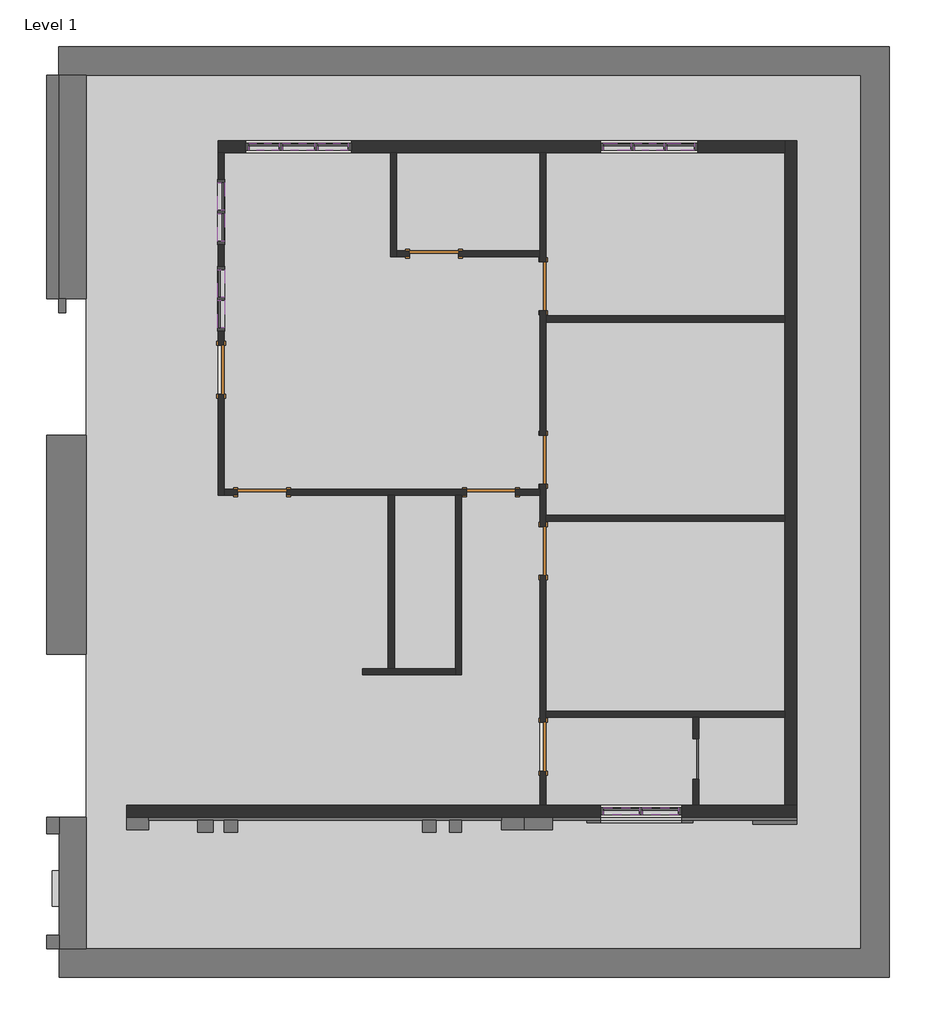
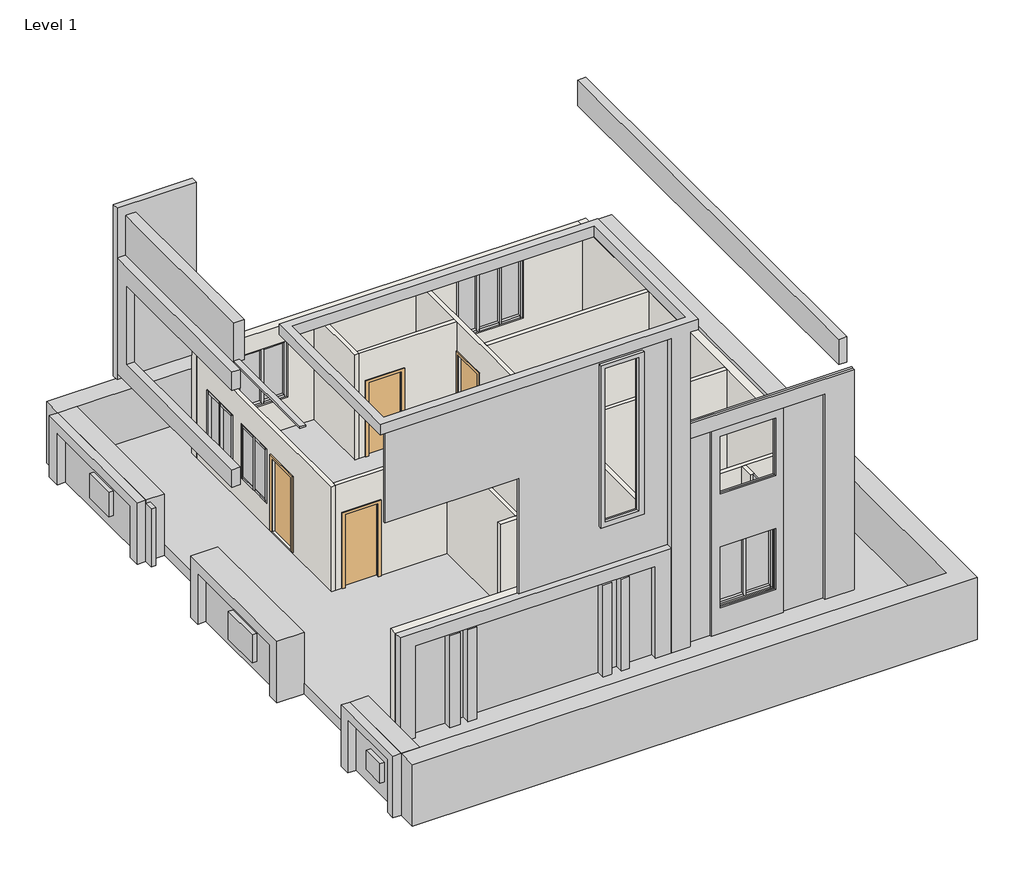
# One storey: 41 members, 15 walls, 13 plates, 8 doors, 7 proxies.
"""IFC4 building model written with IfcOpenShell, lengths in millimetres."""

from ifc_helpers import new_model, si_unit, frame, origin, origin_with_axes, place, context, project, spatial, polyline, outline, extrude, faceted_brep, transform, mapped, element, save
from components import generic_models_1_generic_models_1_e43304c4, generic_models_10_generic_models_10_cbb95902, generic_models_3_generic_models_3_0e3346f0, generic_models_4_generic_models_4_c94f5d84, generic_models_5_generic_models_5_fcb812c2, generic_models_6_generic_models_6_7d9998ff, generic_models_8_generic_models_8_478b8fa0, door_305aa2a5, door_e5f9f3c4, member_0b7646a3, member_1fe8360d, member_921b0d60, member_90febb00, member_2e0784aa, member_a400357f, member_a980948f, member_6f432376, member_c6b50b9a, member_293a584d, member_16047d0f, member_00baf460, member_c33c434a, member_eeabd68d, member_85079546, system_panel_glazed_353c4472, system_panel_glazed_f9beff23, system_panel_glazed_2aec2d59, system_panel_glazed_df895792, system_panel_glazed_ced102d0, system_panel_glazed_0ced4b38, system_panel_glazed_3427ea54, system_panel_glazed_7f229d02

model = new_model("IFC4")

# Units and contexts
model_context = context("Model", 3, world=origin())
ifc_project = project(units=[si_unit("LENGTHUNIT", "METRE", prefix="MILLI")], contexts=[model_context])

# Site, building, storey
site = spatial("IfcSite", under=ifc_project)
building = spatial("IfcBuilding", under=site)
storey = spatial("IfcBuildingStorey", under=building, Name="Level 1", Elevation=0.0)

# Proxies
placement = place(None, origin())
generic_models_1_generic_models_1_shape = generic_models_1_generic_models_1_e43304c4(model_context)
element("IfcBuildingElementProxy", 1, Name="Generic Models 1 : Generic Models 1", ObjectType="Generic Models 1 : Generic Models 1", at=placement, inside=storey, context=model_context, shape_type="MappedRepresentation", body=[
    mapped(generic_models_1_generic_models_1_shape, transform((0.0, 0.0, 0.0), x_axis=(1.0, 0.0, 0.0), y_axis=(0.0, 1.0, 0.0), z_axis=(0.0, 0.0, 1.0))),
])
generic_models_10_generic_models_10_shape = generic_models_10_generic_models_10_cbb95902(model_context)
element("IfcBuildingElementProxy", 2, Name="Generic Models 10 : Generic Models 10", ObjectType="Generic Models 10 : Generic Models 10", at=placement, inside=storey, context=model_context, shape_type="MappedRepresentation", body=[
    mapped(generic_models_10_generic_models_10_shape, transform((0.0, 0.0, 0.0), x_axis=(1.0, 0.0, 0.0), y_axis=(0.0, 1.0, 0.0), z_axis=(0.0, 0.0, 1.0))),
])
generic_models_3_generic_models_3_shape = generic_models_3_generic_models_3_0e3346f0(model_context)
element("IfcBuildingElementProxy", 3, Name="Generic Models 3 : Generic Models 3", ObjectType="Generic Models 3 : Generic Models 3", at=placement, inside=storey, context=model_context, shape_type="MappedRepresentation", body=[
    mapped(generic_models_3_generic_models_3_shape, transform((0.0, 0.0, 0.0), x_axis=(1.0, 0.0, 0.0), y_axis=(0.0, 1.0, 0.0), z_axis=(0.0, 0.0, 1.0))),
])
generic_models_4_generic_models_4_shape = generic_models_4_generic_models_4_c94f5d84(model_context)
element("IfcBuildingElementProxy", 4, Name="Generic Models 4 : Generic Models 4", ObjectType="Generic Models 4 : Generic Models 4", at=placement, inside=storey, context=model_context, shape_type="MappedRepresentation", body=[
    mapped(generic_models_4_generic_models_4_shape, transform((0.0, 0.0, 0.0), x_axis=(1.0, 0.0, 0.0), y_axis=(0.0, 1.0, 0.0), z_axis=(0.0, 0.0, 1.0))),
])
generic_models_5_generic_models_5_shape = generic_models_5_generic_models_5_fcb812c2(model_context)
element("IfcBuildingElementProxy", 5, Name="Generic Models 5 : Generic Models 5", ObjectType="Generic Models 5 : Generic Models 5", at=placement, inside=storey, context=model_context, shape_type="MappedRepresentation", body=[
    mapped(generic_models_5_generic_models_5_shape, transform((0.0, 0.0, 0.0), x_axis=(1.0, 0.0, 0.0), y_axis=(0.0, 1.0, 0.0), z_axis=(0.0, 0.0, 1.0))),
])
generic_models_6_generic_models_6_shape = generic_models_6_generic_models_6_7d9998ff(model_context)
element("IfcBuildingElementProxy", 6, Name="Generic Models 6 : Generic Models 6", ObjectType="Generic Models 6 : Generic Models 6", at=placement, inside=storey, context=model_context, shape_type="MappedRepresentation", body=[
    mapped(generic_models_6_generic_models_6_shape, transform((0.0, 0.0, 0.0), x_axis=(1.0, 0.0, 0.0), y_axis=(0.0, 1.0, 0.0), z_axis=(0.0, 0.0, 1.0))),
])
generic_models_8_generic_models_8_shape = generic_models_8_generic_models_8_478b8fa0(model_context)
element("IfcBuildingElementProxy", 7, Name="Generic Models 8 : Generic Models 8", ObjectType="Generic Models 8 : Generic Models 8", at=placement, inside=storey, context=model_context, shape_type="MappedRepresentation", body=[
    mapped(generic_models_8_generic_models_8_shape, transform((0.0, 0.0, 0.0), x_axis=(1.0, 0.0, 0.0), y_axis=(0.0, 1.0, 0.0), z_axis=(0.0, 0.0, 1.0))),
])

# Doors
door_shape = door_305aa2a5(model_context)
element("IfcDoor", 8, ObjectType="Single-Flush : 36\" x 84\"", at=placement, inside=storey, context=model_context, shape_type="MappedRepresentation", body=[
    mapped(door_shape, transform((-18378.8003587, -5510.4026331, 50.8), x_axis=(0.0, 1.0, 0.0), y_axis=(-1.0, 0.0, 0.0), z_axis=(0.0, 0.0, 1.0))),
])
element("IfcDoor", 9, ObjectType="Single-Flush : 36\" x 84\"", at=placement, inside=storey, context=model_context, shape_type="MappedRepresentation", body=[
    mapped(door_shape, transform((-17616.8003587, -7796.4026331, 0.0), x_axis=(-1.0, 0.0, 0.0), y_axis=(0.0, -1.0, 0.0), z_axis=(0.0, 0.0, 1.0))),
])
element("IfcDoor", 10, ObjectType="Single-Flush : 36\" x 84\"", at=placement, inside=storey, context=model_context, shape_type="MappedRepresentation", body=[
    mapped(door_shape, transform((-14397.3503587, -3338.7026331, 0.0), x_axis=(-1.0, 0.0, 0.0), y_axis=(0.0, -1.0, 0.0), z_axis=(0.0, 0.0, 1.0))),
])
element("IfcDoor", 11, ObjectType="Single-Flush : 36\" x 84\"", at=placement, inside=storey, context=model_context, shape_type="MappedRepresentation", body=[
    mapped(door_shape, transform((-13330.5503587, -7796.4026331, 0.0), x_axis=(-1.0, 0.0, 0.0), y_axis=(0.0, -1.0, 0.0), z_axis=(0.0, 0.0, 1.0))),
])
element("IfcDoor", 12, ObjectType="Single-Flush : 36\" x 84\"", at=placement, inside=storey, context=model_context, shape_type="MappedRepresentation", body=[
    mapped(door_shape, transform((-12359.0003587, -8894.9526331, 0.0), x_axis=(0.0, 1.0, 0.0), y_axis=(-1.0, 0.0, 0.0), z_axis=(0.0, 0.0, 1.0))),
])
element("IfcDoor", 13, ObjectType="Single-Flush : 36\" x 84\"", at=placement, inside=storey, context=model_context, shape_type="MappedRepresentation", body=[
    mapped(door_shape, transform((-12359.0003587, -12552.5526331, 76.2), x_axis=(0.0, 1.0, 0.0), y_axis=(-1.0, 0.0, 0.0), z_axis=(0.0, 0.0, 1.0))),
])
door_2_shape = door_e5f9f3c4(model_context)
element("IfcDoor", 14, ObjectType="Single-Flush : 36\" x 84\"", at=placement, inside=storey, context=model_context, shape_type="MappedRepresentation", body=[
    mapped(door_2_shape, transform((-12359.0003587, -3948.3026331, 0.0), x_axis=(0.0, -1.0, 0.0), y_axis=(1.0, 0.0, 0.0), z_axis=(0.0, 0.0, 1.0))),
])
element("IfcDoor", 15, ObjectType="Single-Flush : 36\" x 84\"", at=placement, inside=storey, context=model_context, shape_type="MappedRepresentation", body=[
    mapped(door_2_shape, transform((-12359.0003587, -7186.8026331, 0.0), x_axis=(0.0, -1.0, 0.0), y_axis=(1.0, 0.0, 0.0), z_axis=(0.0, 0.0, 1.0))),
])

# Members
member_shape = member_0b7646a3(model_context)
element("IfcMember", 16, ObjectType="Rectangular Mullion : 2.5\" x 5\" rectangular", at=placement, inside=storey, context=model_context, shape_type="MappedRepresentation", body=[
    mapped(member_shape, transform((-18378.8003587, -2525.9026331, 2289.8702949), x_axis=(0.0, 0.0, 1.0), y_axis=(-1.0, 0.0, 0.0), z_axis=(0.0, -1.0, 0.0))),
])
element("IfcMember", 17, ObjectType="Rectangular Mullion : 2.5\" x 5\" rectangular", at=placement, inside=storey, context=model_context, shape_type="MappedRepresentation", body=[
    mapped(member_shape, transform((-18378.8003587, -3103.7526331, 2289.8702949), x_axis=(0.0, 0.0, 1.0), y_axis=(-1.0, 0.0, 0.0), z_axis=(0.0, -1.0, 0.0))),
])
element("IfcMember", 18, ObjectType="Rectangular Mullion : 2.5\" x 5\" rectangular", at=placement, inside=storey, context=model_context, shape_type="MappedRepresentation", body=[
    mapped(member_shape, transform((-18378.8003587, -4212.3782104, 2289.8702949), x_axis=(0.0, 0.0, 1.0), y_axis=(1.0, 0.0, 0.0), z_axis=(0.0, 1.0, 0.0))),
])
element("IfcMember", 19, ObjectType="Rectangular Mullion : 2.5\" x 5\" rectangular", at=placement, inside=storey, context=model_context, shape_type="MappedRepresentation", body=[
    mapped(member_shape, transform((-18378.8003587, -3634.5282104, 2289.8702949), x_axis=(0.0, 0.0, 1.0), y_axis=(1.0, 0.0, 0.0), z_axis=(0.0, 1.0, 0.0))),
])
element("IfcMember", 20, ObjectType="Rectangular Mullion : 2.5\" x 5\" rectangular", at=placement, inside=storey, context=model_context, shape_type="MappedRepresentation", body=[
    mapped(member_shape, transform((-10714.3503587, -1338.4526331, 2669.0215701), x_axis=(0.0, 0.0, 1.0), y_axis=(0.0, -1.0, 0.0), z_axis=(1.0, 0.0, 0.0))),
])
element("IfcMember", 21, ObjectType="Rectangular Mullion : 2.5\" x 5\" rectangular", at=placement, inside=storey, context=model_context, shape_type="MappedRepresentation", body=[
    mapped(member_shape, transform((-9526.9003587, -1338.4526331, 2669.0215701), x_axis=(0.0, 0.0, 1.0), y_axis=(0.0, -1.0, 0.0), z_axis=(1.0, 0.0, 0.0))),
])
member_2_shape = member_1fe8360d(model_context)
element("IfcMember", 22, ObjectType="Rectangular Mullion : 2.5\" x 5\" rectangular", at=placement, inside=storey, context=model_context, shape_type="MappedRepresentation", body=[
    mapped(member_2_shape, transform((-18378.8003587, -2557.6526331, 812.6731894), x_axis=(0.0, -1.0, 0.0), y_axis=(-1.0, 0.0, 0.0), z_axis=(0.0, 0.0, -1.0))),
])
element("IfcMember", 23, ObjectType="Rectangular Mullion : 2.5\" x 5\" rectangular", at=placement, inside=storey, context=model_context, shape_type="MappedRepresentation", body=[
    mapped(member_shape, transform((-18378.8003587, -2589.4026331, 812.6731894), x_axis=(0.0, 0.0, -1.0), y_axis=(-1.0, 0.0, 0.0), z_axis=(0.0, 1.0, 0.0))),
])
element("IfcMember", 24, ObjectType="Rectangular Mullion : 2.5\" x 5\" rectangular", at=placement, inside=storey, context=model_context, shape_type="MappedRepresentation", body=[
    mapped(member_shape, transform((-18378.8003587, -2011.5526331, 812.6731894), x_axis=(0.0, 0.0, -1.0), y_axis=(-1.0, 0.0, 0.0), z_axis=(0.0, 1.0, 0.0))),
])
element("IfcMember", 25, ObjectType="Rectangular Mullion : 2.5\" x 5\" rectangular", at=placement, inside=storey, context=model_context, shape_type="MappedRepresentation", body=[
    mapped(member_shape, transform((-18378.8003587, -4148.8782104, 718.4753468), x_axis=(0.0, 0.0, -1.0), y_axis=(1.0, 0.0, 0.0), z_axis=(0.0, -1.0, 0.0))),
])
element("IfcMember", 26, ObjectType="Rectangular Mullion : 2.5\" x 5\" rectangular", at=placement, inside=storey, context=model_context, shape_type="MappedRepresentation", body=[
    mapped(member_shape, transform((-18378.8003587, -4726.7282104, 718.4753468), x_axis=(0.0, 0.0, -1.0), y_axis=(1.0, 0.0, 0.0), z_axis=(0.0, -1.0, 0.0))),
])
element("IfcMember", 27, ObjectType="Rectangular Mullion : 2.5\" x 5\" rectangular", at=placement, inside=storey, context=model_context, shape_type="MappedRepresentation", body=[
    mapped(member_shape, transform((-10041.2503587, -1338.4526331, 927.2562283), x_axis=(0.0, 0.0, -1.0), y_axis=(0.0, -1.0, 0.0), z_axis=(-1.0, 0.0, 0.0))),
])
element("IfcMember", 28, ObjectType="Rectangular Mullion : 2.5\" x 5\" rectangular", at=placement, inside=storey, context=model_context, shape_type="MappedRepresentation", body=[
    mapped(member_shape, transform((-11228.7003587, -1338.4526331, 927.2562283), x_axis=(0.0, 0.0, -1.0), y_axis=(0.0, -1.0, 0.0), z_axis=(-1.0, 0.0, 0.0))),
])
member_3_shape = member_921b0d60(model_context)
element("IfcMember", 29, ObjectType="Rectangular Mullion : 2.5\" x 5\" rectangular", at=placement, inside=storey, context=model_context, shape_type="MappedRepresentation", body=[
    mapped(member_3_shape, transform((-18378.8003587, -3167.2526331, 812.6731894), x_axis=(0.0, -1.0, 0.0), y_axis=(-1.0, 0.0, 0.0), z_axis=(0.0, 0.0, -1.0))),
])
element("IfcMember", 30, ObjectType="Rectangular Mullion : 2.5\" x 5\" rectangular", at=placement, inside=storey, context=model_context, shape_type="MappedRepresentation", body=[
    mapped(member_3_shape, transform((-18378.8003587, -1948.0526331, 2289.8702949), x_axis=(0.0, 1.0, 0.0), y_axis=(-1.0, 0.0, 0.0), z_axis=(0.0, 0.0, 1.0))),
])
member_4_shape = member_90febb00(model_context)
element("IfcMember", 31, ObjectType="Rectangular Mullion : 2.5\" x 5\" rectangular", at=placement, inside=storey, context=model_context, shape_type="MappedRepresentation", body=[
    mapped(member_4_shape, transform((-18378.8003587, -4180.6282104, 718.4753468), x_axis=(0.0, 1.0, 0.0), y_axis=(1.0, 0.0, 0.0), z_axis=(0.0, 0.0, -1.0))),
])
member_5_shape = member_2e0784aa(model_context)
element("IfcMember", 32, ObjectType="Rectangular Mullion : 2.5\" x 5\" rectangular", at=placement, inside=storey, context=model_context, shape_type="MappedRepresentation", body=[
    mapped(member_5_shape, transform((-18378.8003587, -4790.2282104, 2289.8702949), x_axis=(0.0, -1.0, 0.0), y_axis=(1.0, 0.0, 0.0), z_axis=(0.0, 0.0, 1.0))),
])
element("IfcMember", 33, ObjectType="Rectangular Mullion : 2.5\" x 5\" rectangular", at=placement, inside=storey, context=model_context, shape_type="MappedRepresentation", body=[
    mapped(member_5_shape, transform((-18378.8003587, -3571.0282104, 718.4753468), x_axis=(0.0, 1.0, 0.0), y_axis=(1.0, 0.0, 0.0), z_axis=(0.0, 0.0, -1.0))),
])
member_6_shape = member_a400357f(model_context)
element("IfcMember", 34, ObjectType="Rectangular Mullion : 2.5\" x 5\" rectangular", at=placement, inside=storey, context=model_context, shape_type="MappedRepresentation", body=[
    mapped(member_6_shape, transform((-16632.5503587, -1338.4526331, 2544.0832428), x_axis=(0.0, 0.0, 1.0), y_axis=(0.0, -1.0, 0.0), z_axis=(1.0, 0.0, 0.0))),
])
element("IfcMember", 35, ObjectType="Rectangular Mullion : 2.5\" x 5\" rectangular", at=placement, inside=storey, context=model_context, shape_type="MappedRepresentation", body=[
    mapped(member_6_shape, transform((-17229.4503587, -1338.4526331, 900.2328231), x_axis=(0.0, 0.0, -1.0), y_axis=(0.0, -1.0, 0.0), z_axis=(-1.0, 0.0, 0.0))),
])
member_7_shape = member_a980948f(model_context)
element("IfcMember", 36, ObjectType="Rectangular Mullion : 2.5\" x 5\" rectangular", at=placement, inside=storey, context=model_context, shape_type="MappedRepresentation", body=[
    mapped(member_7_shape, transform((-10104.7503587, -1338.4526331, 2669.0215701), x_axis=(0.0, 0.0, 1.0), y_axis=(0.0, -1.0, 0.0), z_axis=(1.0, 0.0, 0.0))),
])
element("IfcMember", 37, ObjectType="Rectangular Mullion : 2.5\" x 5\" rectangular", at=placement, inside=storey, context=model_context, shape_type="MappedRepresentation", body=[
    mapped(member_7_shape, transform((-10650.8503587, -1338.4526331, 927.2562283), x_axis=(0.0, 0.0, -1.0), y_axis=(0.0, -1.0, 0.0), z_axis=(-1.0, 0.0, 0.0))),
])
member_8_shape = member_6f432376(model_context)
element("IfcMember", 38, ObjectType="Rectangular Mullion : 2.5\" x 5\" rectangular", at=placement, inside=storey, context=model_context, shape_type="MappedRepresentation", body=[
    mapped(member_8_shape, transform((-17292.9503587, -1338.4526331, 2544.0832428), x_axis=(0.0, 0.0, 1.0), y_axis=(0.0, -1.0, 0.0), z_axis=(1.0, 0.0, 0.0))),
])
element("IfcMember", 39, ObjectType="Rectangular Mullion : 2.5\" x 5\" rectangular", at=placement, inside=storey, context=model_context, shape_type="MappedRepresentation", body=[
    mapped(member_8_shape, transform((-16003.9003587, -1338.4526331, 2544.0832428), x_axis=(0.0, 0.0, 1.0), y_axis=(0.0, -1.0, 0.0), z_axis=(1.0, 0.0, 0.0))),
])
element("IfcMember", 40, ObjectType="Rectangular Mullion : 2.5\" x 5\" rectangular", at=placement, inside=storey, context=model_context, shape_type="MappedRepresentation", body=[
    mapped(member_8_shape, transform((-16569.0503587, -1338.4526331, 900.2328231), x_axis=(0.0, 0.0, -1.0), y_axis=(0.0, -1.0, 0.0), z_axis=(-1.0, 0.0, 0.0))),
])
element("IfcMember", 41, ObjectType="Rectangular Mullion : 2.5\" x 5\" rectangular", at=placement, inside=storey, context=model_context, shape_type="MappedRepresentation", body=[
    mapped(member_8_shape, transform((-17858.1003587, -1338.4526331, 900.2328231), x_axis=(0.0, 0.0, -1.0), y_axis=(0.0, -1.0, 0.0), z_axis=(-1.0, 0.0, 0.0))),
])
member_9_shape = member_c6b50b9a(model_context)
element("IfcMember", 42, ObjectType="Rectangular Mullion : 2.5\" x 5\" rectangular", at=placement, inside=storey, context=model_context, shape_type="MappedRepresentation", body=[
    mapped(member_9_shape, transform((-10682.6003587, -1338.4526331, 927.2562283), x_axis=(1.0, 0.0, 0.0), y_axis=(0.0, -1.0, 0.0), z_axis=(0.0, 0.0, -1.0))),
])
element("IfcMember", 43, ObjectType="Rectangular Mullion : 2.5\" x 5\" rectangular", at=placement, inside=storey, context=model_context, shape_type="MappedRepresentation", body=[
    mapped(member_9_shape, transform((-10073.0003587, -1338.4526331, 927.2562283), x_axis=(1.0, 0.0, 0.0), y_axis=(0.0, -1.0, 0.0), z_axis=(0.0, 0.0, -1.0))),
])
member_10_shape = member_293a584d(model_context)
element("IfcMember", 44, ObjectType="Rectangular Mullion : 2.5\" x 5\" rectangular", at=placement, inside=storey, context=model_context, shape_type="MappedRepresentation", body=[
    mapped(member_10_shape, transform((-11292.2003587, -1338.4526331, 2669.0215701), x_axis=(-1.0, 0.0, 0.0), y_axis=(0.0, -1.0, 0.0), z_axis=(0.0, 0.0, 1.0))),
])
element("IfcMember", 45, ObjectType="Rectangular Mullion : 2.5\" x 5\" rectangular", at=placement, inside=storey, context=model_context, shape_type="MappedRepresentation", body=[
    mapped(member_10_shape, transform((-9463.4003587, -1338.4526331, 927.2562283), x_axis=(1.0, 0.0, 0.0), y_axis=(0.0, -1.0, 0.0), z_axis=(0.0, 0.0, -1.0))),
])
member_11_shape = member_16047d0f(model_context)
element("IfcMember", 46, ObjectType="Rectangular Mullion : 2.5\" x 5\" rectangular", at=placement, inside=storey, context=model_context, shape_type="MappedRepresentation", body=[
    mapped(member_11_shape, transform((-16600.8003587, -1338.4526331, 900.2328231), x_axis=(1.0, 0.0, 0.0), y_axis=(0.0, -1.0, 0.0), z_axis=(0.0, 0.0, -1.0))),
])
element("IfcMember", 47, ObjectType="Rectangular Mullion : 2.5\" x 5\" rectangular", at=placement, inside=storey, context=model_context, shape_type="MappedRepresentation", body=[
    mapped(member_11_shape, transform((-17261.2003587, -1338.4526331, 900.2328231), x_axis=(1.0, 0.0, 0.0), y_axis=(0.0, -1.0, 0.0), z_axis=(0.0, 0.0, -1.0))),
])
member_12_shape = member_00baf460(model_context)
element("IfcMember", 48, ObjectType="Rectangular Mullion : 2.5\" x 5\" rectangular", at=placement, inside=storey, context=model_context, shape_type="MappedRepresentation", body=[
    mapped(member_12_shape, transform((-17921.6003587, -1338.4526331, 2544.0832428), x_axis=(-1.0, 0.0, 0.0), y_axis=(0.0, -1.0, 0.0), z_axis=(0.0, 0.0, 1.0))),
])
element("IfcMember", 49, ObjectType="Rectangular Mullion : 2.5\" x 5\" rectangular", at=placement, inside=storey, context=model_context, shape_type="MappedRepresentation", body=[
    mapped(member_12_shape, transform((-15940.4003587, -1338.4526331, 900.2328231), x_axis=(1.0, 0.0, 0.0), y_axis=(0.0, -1.0, 0.0), z_axis=(0.0, 0.0, -1.0))),
])
member_13_shape = member_c33c434a(model_context)
element("IfcMember", 50, ObjectType="Rectangular Mullion : 2.5\" x 5\" rectangular", at=placement, inside=storey, context=model_context, shape_type="MappedRepresentation", body=[
    mapped(member_13_shape, transform((-10561.9503587, -13759.0526331, 2511.49538), x_axis=(0.0, 0.0, 1.0), y_axis=(0.0, -1.0, 0.0), z_axis=(1.0, 0.0, 0.0))),
])
element("IfcMember", 51, ObjectType="Rectangular Mullion : 2.5\" x 5\" rectangular", at=placement, inside=storey, context=model_context, shape_type="MappedRepresentation", body=[
    mapped(member_13_shape, transform((-9831.7003587, -13759.0526331, 2511.49538), x_axis=(0.0, 0.0, 1.0), y_axis=(0.0, -1.0, 0.0), z_axis=(1.0, 0.0, 0.0))),
])
element("IfcMember", 52, ObjectType="Rectangular Mullion : 2.5\" x 5\" rectangular", at=placement, inside=storey, context=model_context, shape_type="MappedRepresentation", body=[
    mapped(member_13_shape, transform((-10498.4503587, -13759.0526331, 739.995359), x_axis=(0.0, 0.0, -1.0), y_axis=(0.0, -1.0, 0.0), z_axis=(-1.0, 0.0, 0.0))),
])
element("IfcMember", 53, ObjectType="Rectangular Mullion : 2.5\" x 5\" rectangular", at=placement, inside=storey, context=model_context, shape_type="MappedRepresentation", body=[
    mapped(member_13_shape, transform((-11228.7003587, -13759.0526331, 739.995359), x_axis=(0.0, 0.0, -1.0), y_axis=(0.0, -1.0, 0.0), z_axis=(-1.0, 0.0, 0.0))),
])
member_14_shape = member_eeabd68d(model_context)
element("IfcMember", 54, ObjectType="Rectangular Mullion : 2.5\" x 5\" rectangular", at=placement, inside=storey, context=model_context, shape_type="MappedRepresentation", body=[
    mapped(member_14_shape, transform((-10530.2003587, -13759.0526331, 739.995359), x_axis=(1.0, 0.0, 0.0), y_axis=(0.0, -1.0, 0.0), z_axis=(0.0, 0.0, -1.0))),
])
member_15_shape = member_85079546(model_context)
element("IfcMember", 55, ObjectType="Rectangular Mullion : 2.5\" x 5\" rectangular", at=placement, inside=storey, context=model_context, shape_type="MappedRepresentation", body=[
    mapped(member_15_shape, transform((-9768.2003587, -13759.0526331, 739.995359), x_axis=(1.0, 0.0, 0.0), y_axis=(0.0, -1.0, 0.0), z_axis=(0.0, 0.0, -1.0))),
])
element("IfcMember", 56, ObjectType="Rectangular Mullion : 2.5\" x 5\" rectangular", at=placement, inside=storey, context=model_context, shape_type="MappedRepresentation", body=[
    mapped(member_15_shape, transform((-11292.2003587, -13759.0526331, 2511.49538), x_axis=(-1.0, 0.0, 0.0), y_axis=(0.0, -1.0, 0.0), z_axis=(0.0, 0.0, 1.0))),
])

# Plates
system_panel_glazed_shape = system_panel_glazed_353c4472(model_context)
element("IfcPlate", 57, ObjectType="System Panel : Glazed", at=placement, inside=storey, context=model_context, shape_type="MappedRepresentation", body=[
    mapped(system_panel_glazed_shape, transform((-9501.5003587, -12781.1526331, 0.0), x_axis=(0.0, -1.0, 0.0), y_axis=(1.0, 0.0, 0.0), z_axis=(0.0, 0.0, 1.0))),
])
system_panel_glazed_2_shape = system_panel_glazed_f9beff23(model_context)
element("IfcPlate", 58, ObjectType="System Panel : Glazed", at=placement, inside=storey, context=model_context, shape_type="MappedRepresentation", body=[
    mapped(system_panel_glazed_2_shape, transform((-18378.8003587, -2268.7276331, 876.1731894), x_axis=(0.0, -1.0, 0.0), y_axis=(1.0, 0.0, 0.0), z_axis=(0.0, 0.0, 1.0))),
])
element("IfcPlate", 59, ObjectType="System Panel : Glazed", at=placement, inside=storey, context=model_context, shape_type="MappedRepresentation", body=[
    mapped(system_panel_glazed_2_shape, transform((-18378.8003587, -2846.5776331, 876.1731894), x_axis=(0.0, -1.0, 0.0), y_axis=(1.0, 0.0, 0.0), z_axis=(0.0, 0.0, 1.0))),
])
system_panel_glazed_3_shape = system_panel_glazed_2aec2d59(model_context)
element("IfcPlate", 60, ObjectType="System Panel : Glazed", at=placement, inside=storey, context=model_context, shape_type="MappedRepresentation", body=[
    mapped(system_panel_glazed_3_shape, transform((-18378.8003587, -4469.5532104, 781.9753468), x_axis=(0.0, 1.0, 0.0), y_axis=(-1.0, 0.0, 0.0), z_axis=(0.0, 0.0, 1.0))),
])
element("IfcPlate", 61, ObjectType="System Panel : Glazed", at=placement, inside=storey, context=model_context, shape_type="MappedRepresentation", body=[
    mapped(system_panel_glazed_3_shape, transform((-18378.8003587, -3891.7032104, 781.9753468), x_axis=(0.0, 1.0, 0.0), y_axis=(-1.0, 0.0, 0.0), z_axis=(0.0, 0.0, 1.0))),
])
system_panel_glazed_4_shape = system_panel_glazed_df895792(model_context)
element("IfcPlate", 62, ObjectType="System Panel : Glazed", at=placement, inside=storey, context=model_context, shape_type="MappedRepresentation", body=[
    mapped(system_panel_glazed_4_shape, transform((-10971.5253587, -1338.4526331, 990.7562283), x_axis=(1.0, 0.0, 0.0), y_axis=(0.0, 1.0, 0.0), z_axis=(0.0, 0.0, 1.0))),
])
element("IfcPlate", 63, ObjectType="System Panel : Glazed", at=placement, inside=storey, context=model_context, shape_type="MappedRepresentation", body=[
    mapped(system_panel_glazed_4_shape, transform((-9784.0753587, -1338.4526331, 990.7562283), x_axis=(1.0, 0.0, 0.0), y_axis=(0.0, 1.0, 0.0), z_axis=(0.0, 0.0, 1.0))),
])
system_panel_glazed_5_shape = system_panel_glazed_ced102d0(model_context)
element("IfcPlate", 64, ObjectType="System Panel : Glazed", at=placement, inside=storey, context=model_context, shape_type="MappedRepresentation", body=[
    mapped(system_panel_glazed_5_shape, transform((-10377.8003587, -1338.4526331, 990.7562283), x_axis=(1.0, 0.0, 0.0), y_axis=(0.0, 1.0, 0.0), z_axis=(0.0, 0.0, 1.0))),
])
system_panel_glazed_6_shape = system_panel_glazed_0ced4b38(model_context)
element("IfcPlate", 65, ObjectType="System Panel : Glazed", at=placement, inside=storey, context=model_context, shape_type="MappedRepresentation", body=[
    mapped(system_panel_glazed_6_shape, transform((-17575.5253587, -1338.4526331, 963.7328231), x_axis=(1.0, 0.0, 0.0), y_axis=(0.0, 1.0, 0.0), z_axis=(0.0, 0.0, 1.0))),
])
element("IfcPlate", 66, ObjectType="System Panel : Glazed", at=placement, inside=storey, context=model_context, shape_type="MappedRepresentation", body=[
    mapped(system_panel_glazed_6_shape, transform((-16286.4753587, -1338.4526331, 963.7328231), x_axis=(1.0, 0.0, 0.0), y_axis=(0.0, 1.0, 0.0), z_axis=(0.0, 0.0, 1.0))),
])
system_panel_glazed_7_shape = system_panel_glazed_3427ea54(model_context)
element("IfcPlate", 67, ObjectType="System Panel : Glazed", at=placement, inside=storey, context=model_context, shape_type="MappedRepresentation", body=[
    mapped(system_panel_glazed_7_shape, transform((-16931.0003587, -1338.4526331, 963.7328231), x_axis=(1.0, 0.0, 0.0), y_axis=(0.0, 1.0, 0.0), z_axis=(0.0, 0.0, 1.0))),
])
system_panel_glazed_8_shape = system_panel_glazed_7f229d02(model_context)
element("IfcPlate", 68, ObjectType="System Panel : Glazed", at=placement, inside=storey, context=model_context, shape_type="MappedRepresentation", body=[
    mapped(system_panel_glazed_8_shape, transform((-10895.3253587, -13759.0526331, 803.495359), x_axis=(1.0, 0.0, 0.0), y_axis=(0.0, 1.0, 0.0), z_axis=(0.0, 0.0, 1.0))),
])
element("IfcPlate", 69, ObjectType="System Panel : Glazed", at=placement, inside=storey, context=model_context, shape_type="MappedRepresentation", body=[
    mapped(system_panel_glazed_8_shape, transform((-10165.0753587, -13759.0526331, 803.495359), x_axis=(1.0, 0.0, 0.0), y_axis=(0.0, 1.0, 0.0), z_axis=(0.0, 0.0, 1.0))),
])

# Walls
element("IfcWall", 70, ObjectType="4.5\"", at=placement, inside=storey, context=model_context, shape_type="Brep", body=[
    faceted_brep([(-18435.9503587, -1452.7526331, 0.0), (-18435.9503587, -7853.5526331, 0.0), (-18435.9503587, -7853.5526331, 3048.0), (-18435.9503587, -1452.7526331, 3048.0), (-18435.9503587, -5967.6026331, 50.8), (-18435.9503587, -5053.2026331, 50.8), (-18435.9503587, -5053.2026331, 2184.4), (-18435.9503587, -5967.6026331, 2184.4), (-18435.9503587, -4790.2282104, 2289.8702949), (-18435.9503587, -4790.2282104, 718.4753468), (-18435.9503587, -3571.0282104, 718.4753468), (-18435.9503587, -3571.0282104, 2289.8702949), (-18435.9503587, -1948.0526331, 812.6731894), (-18435.9503587, -1948.0526331, 2289.8702949), (-18435.9503587, -3167.2526331, 2289.8702949), (-18435.9503587, -3167.2526331, 812.6731894), (-18321.6503587, -7853.5526331, 0.0), (-18321.6503587, -7739.2526331, 0.0), (-18321.6503587, -1452.7526331, 0.0), (-18321.6503587, -1452.7526331, 3048.0), (-18321.6503587, -7739.2526331, 3048.0), (-18321.6503587, -7853.5526331, 3048.0), (-18321.6503587, -5967.6026331, 50.8), (-18321.6503587, -5967.6026331, 2184.4), (-18321.6503587, -5053.2026331, 2184.4), (-18321.6503587, -5053.2026331, 50.8), (-18321.6503587, -4790.2282104, 718.4753468), (-18321.6503587, -4790.2282104, 2289.8702949), (-18321.6503587, -3571.0282104, 2289.8702949), (-18321.6503587, -3571.0282104, 718.4753468), (-18321.6503587, -1948.0526331, 2289.8702949), (-18321.6503587, -1948.0526331, 812.6731894), (-18321.6503587, -3167.2526331, 812.6731894), (-18321.6503587, -3167.2526331, 2289.8702949)], [[[0, 1, 2, 3], [4, 5, 6, 7], [8, 9, 10, 11], [12, 13, 14, 15]], [[16, 17, 18, 19, 20, 21], [22, 23, 24, 25], [26, 27, 28, 29], [30, 31, 32, 33]], [[1, 0, 18, 17, 16]], [[3, 2, 21, 20, 19]], [[0, 3, 19, 18]], [[2, 1, 16, 21]], [[5, 4, 22, 25]], [[6, 5, 25, 24]], [[7, 6, 24, 23]], [[4, 7, 23, 22]], [[26, 9, 8, 27]], [[27, 8, 11, 28]], [[10, 29, 28, 11]], [[9, 26, 29, 10]], [[12, 31, 30, 13]], [[13, 30, 33, 14]], [[14, 33, 32, 15]], [[31, 12, 15, 32]]]),
])
element("IfcWall", 71, ObjectType="4.5\"", at=placement, inside=storey, context=model_context, shape_type="Brep", body=[
    faceted_brep([(-12416.1503587, -7644.0026331, 0.0), (-12416.1503587, -7739.2526331, 0.0), (-12416.1503587, -7853.5526331, 0.0), (-12416.1503587, -8437.7526331, 0.0), (-12416.1503587, -8437.7526331, 2133.6), (-12416.1503587, -9352.1526331, 2133.6), (-12416.1503587, -9352.1526331, 0.0), (-12416.1503587, -13644.7526331, 0.0), (-12416.1503587, -13644.7526331, 3048.0), (-12416.1503587, -7853.5526331, 3048.0), (-12416.1503587, -7739.2526331, 3048.0), (-12416.1503587, -3395.8526331, 3048.0), (-12416.1503587, -3281.5526331, 3048.0), (-12416.1503587, -1452.7526331, 3048.0), (-12416.1503587, -1452.7526331, 0.0), (-12416.1503587, -3281.5526331, 0.0), (-12416.1503587, -3395.8526331, 0.0), (-12416.1503587, -3491.1026331, 0.0), (-12416.1503587, -3491.1026331, 2133.6), (-12416.1503587, -4405.5026331, 2133.6), (-12416.1503587, -4405.5026331, 0.0), (-12416.1503587, -6729.6026331, 0.0), (-12416.1503587, -6729.6026331, 2133.6), (-12416.1503587, -7644.0026331, 2133.6), (-12416.1503587, -13009.7526331, 76.2), (-12416.1503587, -12095.3526331, 76.2), (-12416.1503587, -12095.3526331, 2209.8), (-12416.1503587, -13009.7526331, 2209.8), (-12301.8503587, -8437.7526331, 2133.6), (-12301.8503587, -8437.7526331, 0.0), (-12301.8503587, -8342.5026331, 0.0), (-12301.8503587, -8228.2026331, 0.0), (-12301.8503587, -7644.0026331, 0.0), (-12301.8503587, -7644.0026331, 2133.6), (-12301.8503587, -6729.6026331, 2133.6), (-12301.8503587, -6729.6026331, 0.0), (-12301.8503587, -4615.0526331, 0.0), (-12301.8503587, -4500.7526331, 0.0), (-12301.8503587, -4405.5026331, 0.0), (-12301.8503587, -4405.5026331, 2133.6), (-12301.8503587, -3491.1026331, 2133.6), (-12301.8503587, -3491.1026331, 0.0), (-12301.8503587, -1452.7526331, 0.0), (-12301.8503587, -1452.7526331, 3048.0), (-12301.8503587, -4500.7526331, 3048.0), (-12301.8503587, -4615.0526331, 3048.0), (-12301.8503587, -8228.2026331, 3048.0), (-12301.8503587, -8342.5026331, 3048.0), (-12301.8503587, -11885.8026331, 3048.0), (-12301.8503587, -12000.1026331, 3048.0), (-12301.8503587, -13644.7526331, 3048.0), (-12301.8503587, -13644.7526331, 0.0), (-12301.8503587, -12000.1026331, 0.0), (-12301.8503587, -11885.8026331, 0.0), (-12301.8503587, -9352.1526331, 0.0), (-12301.8503587, -9352.1526331, 2133.6), (-12301.8503587, -13009.7526331, 76.2), (-12301.8503587, -13009.7526331, 2209.8), (-12301.8503587, -12095.3526331, 2209.8), (-12301.8503587, -12095.3526331, 76.2)], [[[0, 1, 2, 3, 4, 5, 6, 7, 8, 9, 10, 11, 12, 13, 14, 15, 16, 17, 18, 19, 20, 21, 22, 23], [24, 25, 26, 27]], [[28, 29, 30, 31, 32, 33, 34, 35, 36, 37, 38, 39, 40, 41, 42, 43, 44, 45, 46, 47, 48, 49, 50, 51, 52, 53, 54, 55], [56, 57, 58, 59]], [[17, 16, 15, 14, 42, 41]], [[21, 20, 38, 37, 36, 35]], [[32, 31, 30, 29, 3, 2, 1, 0]], [[54, 53, 52, 51, 7, 6]], [[13, 12, 11, 10, 9, 8, 50, 49, 48, 47, 46, 45, 44, 43]], [[14, 13, 43, 42]], [[8, 7, 51, 50]], [[39, 38, 20, 19]], [[40, 39, 19, 18]], [[41, 40, 18, 17]], [[33, 32, 0, 23]], [[34, 33, 23, 22]], [[35, 34, 22, 21]], [[4, 3, 29, 28]], [[5, 4, 28, 55]], [[6, 5, 55, 54]], [[25, 24, 56, 59]], [[26, 25, 59, 58]], [[27, 26, 58, 57]], [[24, 27, 57, 56]]]),
])
element("IfcWall", 72, ObjectType="4.5\"", at=placement, inside=storey, context=model_context, shape_type="SweptSolid", body=[
    extrude(outline(polyline([(-7844.1503587, -4615.0526331), (-12301.8503587, -4615.0526331), (-12301.8503587, -4500.7526331), (-7844.1503587, -4500.7526331), (-7844.1503587, -4615.0526331)])), origin_with_axes(), (0.0, 0.0, 1.0), 3048.0),
])
element("IfcWall", 73, ObjectType="4.5\"", at=placement, inside=storey, context=model_context, shape_type="Brep", body=[
    faceted_brep([(-15216.5003587, -1452.7526331, 0.0), (-15216.5003587, -3395.8526331, 0.0), (-15216.5003587, -3395.8526331, 3048.0), (-15216.5003587, -1452.7526331, 3048.0), (-15102.2003587, -1452.7526331, 0.0), (-15102.2003587, -1452.7526331, 3048.0), (-15102.2003587, -3281.5526331, 3048.0), (-15102.2003587, -3395.8526331, 3048.0), (-15102.2003587, -3395.8526331, 0.0), (-15102.2003587, -3281.5526331, 0.0)], [[[0, 1, 2, 3]], [[4, 5, 6, 7, 8, 9]], [[1, 0, 4, 9, 8]], [[3, 2, 7, 6, 5]], [[0, 3, 5, 4]], [[2, 1, 8, 7]]]),
])
element("IfcWall", 74, ObjectType="4.5\"", at=placement, inside=storey, context=model_context, shape_type="SweptSolid", body=[
    extrude(outline(polyline([(0.0, -15102.2003587), (0.0, -14854.5503587), (2133.6, -14854.5503587), (2133.6, -13940.1503587), (0.0, -13940.1503587), (0.0, -12416.1503587), (3048.0, -12416.1503587), (3048.0, -15102.2003587), (0.0, -15102.2003587)])), frame((0.0, -3395.8526331, 0.0), z_axis=(0.0, 1.0, 0.0), x_axis=(0.0, 0.0, 1.0)), (0.0, 0.0, 1.0), 114.3),
])
element("IfcWall", 75, ObjectType="4.5\"", at=placement, inside=storey, context=model_context, shape_type="SweptSolid", body=[
    extrude(outline(polyline([(-7844.1503587, -8342.5026331), (-12301.8503587, -8342.5026331), (-12301.8503587, -8228.2026331), (-7844.1503587, -8228.2026331), (-7844.1503587, -8342.5026331)])), origin_with_axes(), (0.0, 0.0, 1.0), 3048.0),
])
element("IfcWall", 76, ObjectType="4.5\"", at=placement, inside=storey, context=model_context, shape_type="Brep", body=[
    faceted_brep([(-12301.8503587, -12000.1026331, 0.0), (-9558.6503587, -12000.1026331, 0.0), (-9444.3503587, -12000.1026331, 0.0), (-7844.1503587, -12000.1026331, 0.0), (-7844.1503587, -12000.1026331, 3048.0), (-9444.3503587, -12000.1026331, 3048.0), (-9558.6503587, -12000.1026331, 3048.0), (-12301.8503587, -12000.1026331, 3048.0), (-12301.8503587, -11885.8026331, 0.0), (-12301.8503587, -11885.8026331, 3048.0), (-7844.1503587, -11885.8026331, 3048.0), (-7844.1503587, -11885.8026331, 0.0)], [[[0, 1, 2, 3, 4, 5, 6, 7]], [[8, 9, 10, 11]], [[3, 2, 1, 0, 8, 11]], [[7, 6, 5, 4, 10, 9]], [[0, 7, 9, 8]], [[4, 3, 11, 10]]]),
])
element("IfcWall", 77, ObjectType="4.5\"", at=placement, inside=storey, context=model_context, shape_type="Brep", body=[
    faceted_brep([(-17159.6003587, -7853.5526331, 0.0), (-15254.6003587, -7853.5526331, 0.0), (-15140.3003587, -7853.5526331, 0.0), (-13997.3003587, -7853.5526331, 0.0), (-13883.0003587, -7853.5526331, 0.0), (-13787.7503587, -7853.5526331, 0.0), (-13787.7503587, -7853.5526331, 2133.6), (-12873.3503587, -7853.5526331, 2133.6), (-12873.3503587, -7853.5526331, 0.0), (-12416.1503587, -7853.5526331, 0.0), (-12416.1503587, -7853.5526331, 3048.0), (-13883.0003587, -7853.5526331, 3048.0), (-13997.3003587, -7853.5526331, 3048.0), (-15140.3003587, -7853.5526331, 3048.0), (-15254.6003587, -7853.5526331, 3048.0), (-18321.6503587, -7853.5526331, 3048.0), (-18321.6503587, -7853.5526331, 0.0), (-18074.0003587, -7853.5526331, 0.0), (-18074.0003587, -7853.5526331, 2133.6), (-17159.6003587, -7853.5526331, 2133.6), (-13787.7503587, -7739.2526331, 2133.6), (-13787.7503587, -7739.2526331, 0.0), (-17159.6003587, -7739.2526331, 0.0), (-17159.6003587, -7739.2526331, 2133.6), (-18074.0003587, -7739.2526331, 2133.6), (-18074.0003587, -7739.2526331, 0.0), (-18321.6503587, -7739.2526331, 0.0), (-18321.6503587, -7739.2526331, 3048.0), (-12416.1503587, -7739.2526331, 3048.0), (-12416.1503587, -7739.2526331, 0.0), (-12873.3503587, -7739.2526331, 0.0), (-12873.3503587, -7739.2526331, 2133.6)], [[[0, 1, 2, 3, 4, 5, 6, 7, 8, 9, 10, 11, 12, 13, 14, 15, 16, 17, 18, 19]], [[20, 21, 22, 23, 24, 25, 26, 27, 28, 29, 30, 31]], [[26, 25, 17, 16]], [[30, 29, 9, 8]], [[22, 21, 5, 4, 3, 2, 1, 0]], [[15, 14, 13, 12, 11, 10, 28, 27]], [[16, 15, 27, 26]], [[10, 9, 29, 28]], [[18, 17, 25, 24]], [[19, 18, 24, 23]], [[0, 19, 23, 22]], [[6, 5, 21, 20]], [[7, 6, 20, 31]], [[8, 7, 31, 30]]]),
])
element("IfcWall", 78, ObjectType="4.5\"", at=placement, inside=storey, context=model_context, shape_type="Brep", body=[
    faceted_brep([(-13997.3003587, -7853.5526331, 0.0), (-13997.3003587, -11092.0526331, 0.0), (-13997.3003587, -11206.3526331, 0.0), (-13997.3003587, -11206.3526331, 3048.0), (-13997.3003587, -11092.0526331, 3048.0), (-13997.3003587, -7853.5526331, 3048.0), (-13883.0003587, -7853.5526331, 0.0), (-13883.0003587, -7853.5526331, 3048.0), (-13883.0003587, -11206.3526331, 3048.0), (-13883.0003587, -11206.3526331, 0.0)], [[[0, 1, 2, 3, 4, 5]], [[6, 7, 8, 9]], [[2, 1, 0, 6, 9]], [[5, 4, 3, 8, 7]], [[0, 5, 7, 6]], [[3, 2, 9, 8]]]),
])
element("IfcWall", 79, ObjectType="4.5\"", at=placement, inside=storey, context=model_context, shape_type="Brep", body=[
    faceted_brep([(-13997.3003587, -11092.0526331, 0.0), (-15140.3003587, -11092.0526331, 0.0), (-15254.6003587, -11092.0526331, 0.0), (-15737.2003587, -11092.0526331, 0.0), (-15737.2003587, -11092.0526331, 3048.0), (-15254.6003587, -11092.0526331, 3048.0), (-15140.3003587, -11092.0526331, 3048.0), (-13997.3003587, -11092.0526331, 3048.0), (-13997.3003587, -11206.3526331, 0.0), (-13997.3003587, -11206.3526331, 3048.0), (-15737.2003587, -11206.3526331, 3048.0), (-15737.2003587, -11206.3526331, 0.0)], [[[0, 1, 2, 3, 4, 5, 6, 7]], [[8, 9, 10, 11]], [[3, 2, 1, 0, 8, 11]], [[4, 3, 11, 10]], [[7, 6, 5, 4, 10, 9]], [[0, 7, 9, 8]]]),
])
element("IfcWall", 80, ObjectType="4.5\"", at=placement, inside=storey, context=model_context, shape_type="SweptSolid", body=[
    extrude(outline(polyline([(-15140.3003587, -7853.5526331), (-15140.3003587, -11092.0526331), (-15254.6003587, -11092.0526331), (-15254.6003587, -7853.5526331), (-15140.3003587, -7853.5526331)])), origin_with_axes(), (0.0, 0.0, 1.0), 3048.0),
])
element("IfcWall", 81, ObjectType="4.5\"", at=placement, inside=storey, context=model_context, shape_type="SweptSolid", body=[
    extrude(outline(polyline([(-9444.3503587, -13644.7526331), (-9558.6503587, -13644.7526331), (-9558.6503587, -13162.1526331), (-9444.3503587, -13162.1526331), (-9444.3503587, -13644.7526331)])), origin_with_axes(), (0.0, 0.0, 1.0), 3048.0),
    extrude(outline(polyline([(-9558.6503587, -12000.1026331), (-9444.3503587, -12000.1026331), (-9444.3503587, -12400.1526331), (-9558.6503587, -12400.1526331), (-9558.6503587, -12000.1026331)])), origin_with_axes(), (0.0, 0.0, 1.0), 3048.0),
])
element("IfcWall", 82, ObjectType="9\"", at=placement, inside=storey, context=model_context, shape_type="Brep", body=[
    faceted_brep([(-20150.4503587, -13873.3526331, 0.0), (-7615.5503587, -13873.3526331, 0.0), (-7615.5503587, -13873.3526331, 3048.0), (-20150.4503587, -13873.3526331, 3048.0), (-11292.2003587, -13873.3526331, 739.995359), (-11292.2003587, -13873.3526331, 2511.49538), (-9768.2003587, -13873.3526331, 2511.49538), (-9768.2003587, -13873.3526331, 739.995359), (-7615.5503587, -13644.7526331, 0.0), (-7844.1503587, -13644.7526331, 0.0), (-9444.3503587, -13644.7526331, 0.0), (-9558.6503587, -13644.7526331, 0.0), (-12301.8503587, -13644.7526331, 0.0), (-12416.1503587, -13644.7526331, 0.0), (-20150.4503587, -13644.7526331, 0.0), (-20150.4503587, -13644.7526331, 3048.0), (-12416.1503587, -13644.7526331, 3048.0), (-12301.8503587, -13644.7526331, 3048.0), (-9558.6503587, -13644.7526331, 3048.0), (-9444.3503587, -13644.7526331, 3048.0), (-7844.1503587, -13644.7526331, 3048.0), (-7615.5503587, -13644.7526331, 3048.0), (-11292.2003587, -13644.7526331, 2511.49538), (-11292.2003587, -13644.7526331, 739.995359), (-9768.2003587, -13644.7526331, 739.995359), (-9768.2003587, -13644.7526331, 2511.49538)], [[[0, 1, 2, 3], [4, 5, 6, 7]], [[8, 9, 10, 11, 12, 13, 14, 15, 16, 17, 18, 19, 20, 21], [22, 23, 24, 25]], [[1, 0, 14, 13, 12, 11, 10, 9, 8]], [[3, 2, 21, 20, 19, 18, 17, 16, 15]], [[0, 3, 15, 14]], [[2, 1, 8, 21]], [[4, 23, 22, 5]], [[5, 22, 25, 6]], [[6, 25, 24, 7]], [[23, 4, 7, 24]]]),
])
element("IfcWall", 83, ObjectType="9\"", at=placement, inside=storey, context=model_context, shape_type="Brep", body=[
    faceted_brep([(-7615.5503587, -13644.7526331, 0.0), (-7615.5503587, -1224.1526331, 0.0), (-7615.5503587, -1224.1526331, 3048.0), (-7615.5503587, -13644.7526331, 3048.0), (-7844.1503587, -13644.7526331, 0.0), (-7844.1503587, -13644.7526331, 3048.0), (-7844.1503587, -12000.1026331, 3048.0), (-7844.1503587, -11885.8026331, 3048.0), (-7844.1503587, -8342.5026331, 3048.0), (-7844.1503587, -8228.2026331, 3048.0), (-7844.1503587, -4615.0526331, 3048.0), (-7844.1503587, -4500.7526331, 3048.0), (-7844.1503587, -1452.7526331, 3048.0), (-7844.1503587, -1224.1526331, 3048.0), (-7844.1503587, -1224.1526331, 0.0), (-7844.1503587, -1452.7526331, 0.0), (-7844.1503587, -4500.7526331, 0.0), (-7844.1503587, -4615.0526331, 0.0), (-7844.1503587, -8228.2026331, 0.0), (-7844.1503587, -8342.5026331, 0.0), (-7844.1503587, -11885.8026331, 0.0), (-7844.1503587, -12000.1026331, 0.0)], [[[0, 1, 2, 3]], [[4, 5, 6, 7, 8, 9, 10, 11, 12, 13, 14, 15, 16, 17, 18, 19, 20, 21]], [[1, 0, 4, 21, 20, 19, 18, 17, 16, 15, 14]], [[3, 2, 13, 12, 11, 10, 9, 8, 7, 6, 5]], [[0, 3, 5, 4]], [[2, 1, 14, 13]]]),
])
element("IfcWall", 84, ObjectType="9\"", at=placement, inside=storey, context=model_context, shape_type="Brep", body=[
    faceted_brep([(-7844.1503587, -1224.1526331, 0.0), (-18435.9503587, -1224.1526331, 0.0), (-18435.9503587, -1224.1526331, 3048.0), (-7844.1503587, -1224.1526331, 3048.0), (-17921.6003587, -1224.1526331, 2544.0832428), (-17921.6003587, -1224.1526331, 900.2328231), (-15940.4003587, -1224.1526331, 900.2328231), (-15940.4003587, -1224.1526331, 2544.0832428), (-11292.2003587, -1224.1526331, 2669.0215701), (-11292.2003587, -1224.1526331, 927.2562283), (-9463.4003587, -1224.1526331, 927.2562283), (-9463.4003587, -1224.1526331, 2669.0215701), (-18435.9503587, -1452.7526331, 0.0), (-18321.6503587, -1452.7526331, 0.0), (-15216.5003587, -1452.7526331, 0.0), (-15102.2003587, -1452.7526331, 0.0), (-12416.1503587, -1452.7526331, 0.0), (-12301.8503587, -1452.7526331, 0.0), (-7844.1503587, -1452.7526331, 0.0), (-7844.1503587, -1452.7526331, 3048.0), (-12301.8503587, -1452.7526331, 3048.0), (-12416.1503587, -1452.7526331, 3048.0), (-15102.2003587, -1452.7526331, 3048.0), (-15216.5003587, -1452.7526331, 3048.0), (-18321.6503587, -1452.7526331, 3048.0), (-18435.9503587, -1452.7526331, 3048.0), (-17921.6003587, -1452.7526331, 900.2328231), (-17921.6003587, -1452.7526331, 2544.0832428), (-15940.4003587, -1452.7526331, 2544.0832428), (-15940.4003587, -1452.7526331, 900.2328231), (-11292.2003587, -1452.7526331, 927.2562283), (-11292.2003587, -1452.7526331, 2669.0215701), (-9463.4003587, -1452.7526331, 2669.0215701), (-9463.4003587, -1452.7526331, 927.2562283)], [[[0, 1, 2, 3], [4, 5, 6, 7], [8, 9, 10, 11]], [[12, 13, 14, 15, 16, 17, 18, 19, 20, 21, 22, 23, 24, 25], [26, 27, 28, 29], [30, 31, 32, 33]], [[1, 0, 18, 17, 16, 15, 14, 13, 12]], [[2, 1, 12, 25]], [[3, 2, 25, 24, 23, 22, 21, 20, 19]], [[0, 3, 19, 18]], [[26, 5, 4, 27]], [[27, 4, 7, 28]], [[28, 7, 6, 29]], [[5, 26, 29, 6]], [[8, 31, 30, 9]], [[31, 8, 11, 32]], [[32, 11, 10, 33]], [[9, 30, 33, 10]]]),
])

save(model, "model.ifc")

# Revit data of these elements
# Type "Single-Flush : 36\" x 84\""
#   Type Mark = "1"
#   Construction Type Id = "MDOOR"
#   Assembly Code = "C1020"
#   Analytic Construction = "Metal"
#   Thickness = 0' - 2"
#   Heat Transfer Coefficient (U) = 0.651978 BTU/(h·ft²·°F)
#   Height = 7' - 0"
#   Trim Projection Ext = 0' - 1"
#   Trim Projection Int = 0' - 1"
#   Trim Width = 0' - 3"
#   Width = 3' - 0"
#   Define Thermal Properties by = 1
#   Define Thermal Properties by = 1
#   Door Material = Door - Panel
#   Frame Material = Door - Frame
#   Visual Light Transmittance = 0
#   Solar Heat Gain Coefficient = 0
#   Function = (empty or 0)
#   Wall Closure = (empty or 0)
# Type "Rectangular Mullion : 2.5\" x 5\" rectangular"
#   built-in parameter 1007304 = 0.416667 (stored number, unit not read)
#   built-in parameter 1007301 = 0.104167 (stored number, unit not read)
#   built-in parameter 1007300 = 0.104167 (stored number, unit not read)
# Type "System Panel : Glazed"
#   Construction Type Id = "GSP4R"
#   Analytic Construction = "1/8 in Pilkington single glazing"
#   Visual Light Transmittance = 0.9
#   Solar Heat Gain Coefficient = 0.86
#   Heat Transfer Coefficient (U) = 1.18115 BTU/(h·ft²·°F)
#   Define Thermal Properties by = 1
# Type "4.5\""
#   Assembly Code = "B2010"
#   Layers, outside or top first: 0' - 4 1/2" no material (function 1)
# Type "9\""
#   Assembly Code = "B2010"
#   Layers, outside or top first: 0' - 9" no material (function 1)
# Element 1 (IfcBuildingElementProxy, "Generic Models 1 : Generic Models 1")
#   Phase Created = New Construction
# Element 2 (IfcBuildingElementProxy, "Generic Models 10 : Generic Models 10")
#   Phase Created = New Construction
# Element 3 (IfcBuildingElementProxy, "Generic Models 3 : Generic Models 3")
#   Phase Created = New Construction
# Element 4 (IfcBuildingElementProxy, "Generic Models 4 : Generic Models 4")
#   Phase Created = New Construction
# Element 5 (IfcBuildingElementProxy, "Generic Models 5 : Generic Models 5")
#   Phase Created = New Construction
# Element 6 (IfcBuildingElementProxy, "Generic Models 6 : Generic Models 6")
#   Phase Created = New Construction
# Element 7 (IfcBuildingElementProxy, "Generic Models 8 : Generic Models 8")
#   Phase Created = New Construction
# Elements 8, 9, 10, 11, 12, 13, 14, 15 (IfcDoor, "Single-Flush : 36\" x 84\"")
#   Phase Created = New Construction
#   Materials on its faces: "Door - Frame", "Door - Panel"
# Elements 16, 17, 18, 19, 20, 21, 22, 23, 24, 25, 26, 27, 28, 29, 30, 31, 32, 33, 34, 35, 36, 37, 38, 39, 40, 41, 42, 43, 44, 45, 46, 47, 48, 49, 50, 51, 52, 53, 54, 55, 56 (IfcMember, "Rectangular Mullion : 2.5\" x 5\" rectangular")
#   Phase Created = New Construction
#   Materials on its faces: "Aluminum"
# Elements 57, 58, 59, 60, 61, 62, 63, 64, 65, 66, 67, 68, 69 (IfcPlate, "System Panel : Glazed")
#   Phase Created = New Construction
#   Materials on its faces: "Glass"
# Elements 70, 71, 72, 73, 74, 75, 76, 77, 78, 79, 80, 81 (IfcWall, "4.5\"")
#   Top Offset = 0' - 0"
#   Base Offset = 0' - 0"
#   Unconnected Height = 10' - 0"
#   wall height = 10' - 0"
#   Phase Created = New Construction
#   Base Constraint = Level 1
#   Materials on its faces: "Default Wall"
# Elements 82, 83, 84 (IfcWall, "9\"")
#   Top Offset = 0' - 0"
#   Base Offset = 0' - 0"
#   Unconnected Height = 10' - 0"
#   wall height = 10' - 0"
#   Phase Created = New Construction
#   Base Constraint = Level 1
#   Materials on its faces: "Default Wall"
# Materials
#   "Door - Panel": class "Wood", colour RGB 210 159 95, transparency 0, Cost = 0
#   "Door - Frame": colour RGB 118 70 51, transparency 0, Cost = 0
#   "Aluminum": class "Metal", colour RGB 247 247 247, transparency 0, Description = "Aluminum 6061", Cost = 0
#   "Glass": class "Glass", colour RGB 0 128 192, transparency 0.75, Description = "Soda Lime Glass", Cost = 0
#   "Default Wall": colour RGB 128 128 128, transparency 0, Cost = 0
